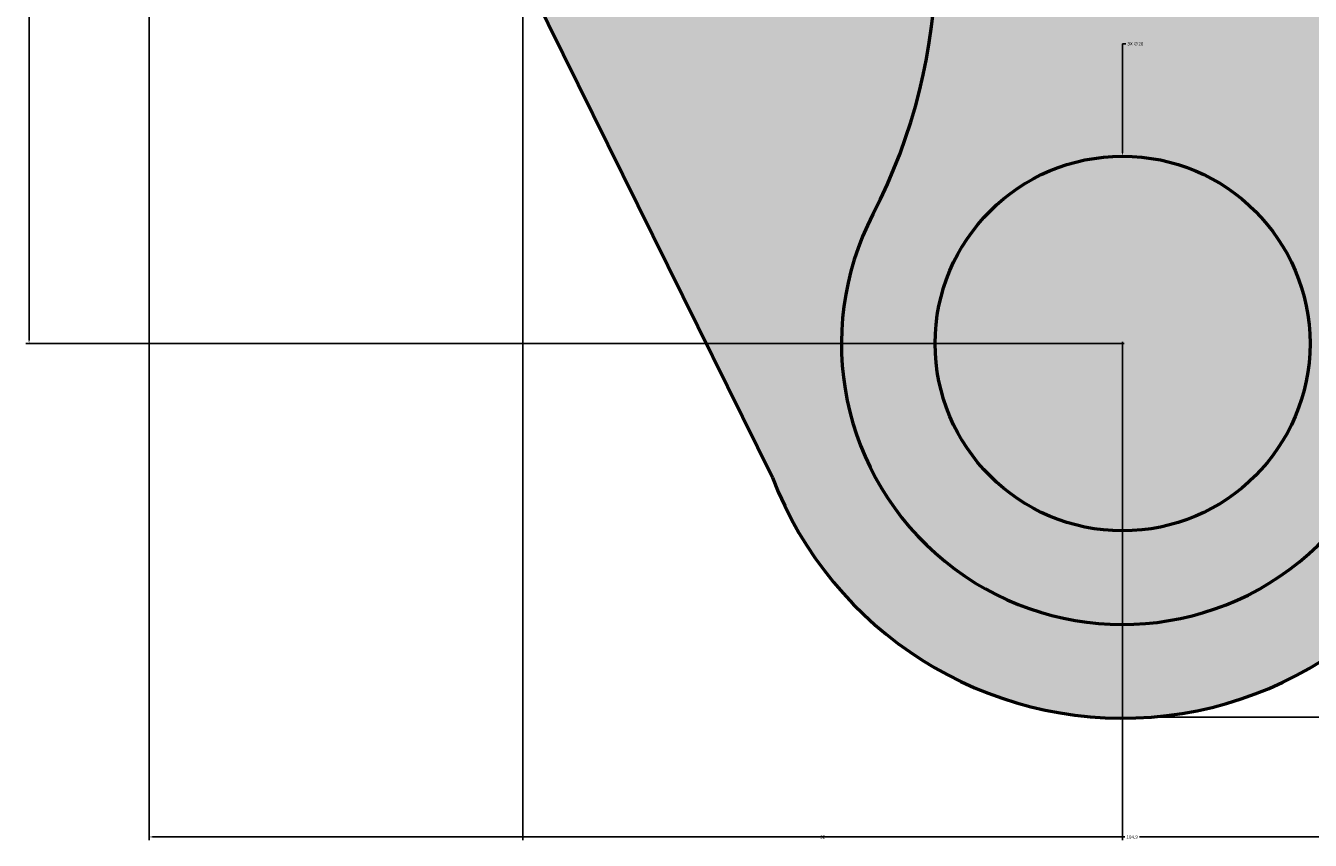
# Model space of a CAD drawing. Units: inches. Extents: x -31 to 87, y -18 to 100.
# Tile 1 of 7: x -31 to 37, y -18 to 25. Entities that reach past the tile are written whole.
import ezdxf

# ---------------------------------------------------------------- set-up
doc = ezdxf.new("R2010")
doc.units = ezdxf.units.IN
doc.header["$MEASUREMENT"] = 0
for name, color, linetype, lineweight in [('M-DIMS', 2, 'Continuous', 18), ('M-HATC', 7, 'Continuous', 18), ('M-OUTL', 4, 'Continuous', 50)]:
    doc.layers.add(name, color=color, linetype=linetype, lineweight=lineweight)
doc.styles.get("Standard").update_dxf_attribs({"font": 'arial.ttf'})
doc.dimstyles.get("Standard").update_dxf_attribs({"dimtxt": 0.18, "dimasz": 0.18, "dimexe": 0.18, "dimexo": 0.0625, "dimgap": 0.09, "dimtad": 0, "dimtih": 1, "dimtoh": 1, "dimdec": 4, "dimzin": 0, "dimdsep": 46, "dimtxsty": 'Standard', "dimcen": 0.09, "dimadec": 0, "dimazin": 0, "dimtfac": 1, "dimtdec": 4, "dimtofl": 0, "dimtmove": 0, "dimatfit": 3, "dimfxl": 1, "dimtolj": 1, "dimtzin": 0, "dimarcsym": 0})

# ---------------------------------------------------------------- blocks, each defined once
blk = doc.blocks.new('*D1')
at = {"layer": 'Defpoints', "color": 0, "transparency": 16777216}
for p in [(-24.622, 75.027), (80.28, 72.235), (80.28, -17.851)]:
    blk.add_point(p, dxfattribs=at)
at = {"layer": 'M-DIMS', "color": 0, "lineweight": -2, "transparency": 16777216}
for p, q in [((-24.622, 74.965), (-24.622, -18.031)), ((80.28, 72.173), (80.28, -18.031)), ((-24.442, -17.851), (27.443, -17.851)), ((80.1, -17.851), (28.214, -17.851))]:
    blk.add_line(p, q, dxfattribs=at)
at = {"layer": 'M-DIMS', "color": 0, "transparency": 16777216}
for points in [[(-24.442, -17.821), (-24.442, -17.881), (-24.622, -17.851)], [(80.1, -17.821), (80.1, -17.881), (80.28, -17.851)]]:
    blk.add_solid(points, dxfattribs=at)
at = {"layer": 'M-DIMS', "color": 0, "transparency": 16777216, "insert": (27.829, -17.851), "char_height": 0.18, "attachment_point": 5}
blk.add_mtext('\\A1;104.9', dxfattribs=at)
blk = doc.blocks.new('*D2')
at = {"layer": 'Defpoints', "color": 0, "transparency": 16777216}
for p in [(60.278, 93.49), (86.68, 93.49), (28.858, -11.451)]:
    blk.add_point(p, dxfattribs=at)
at = {"layer": 'M-DIMS', "color": 0, "lineweight": -2, "transparency": 16777216}
for p, q in [((60.341, 93.49), (86.86, 93.49)), ((86.68, 93.31), (86.68, 41.201)), ((86.68, -11.271), (86.68, 40.838)), ((28.92, -11.451), (86.86, -11.451))]:
    blk.add_line(p, q, dxfattribs=at)
at = {"layer": 'M-DIMS', "color": 0, "transparency": 16777216}
for points in [[(86.65, 93.31), (86.71, 93.31), (86.68, 93.49)], [(86.65, -11.271), (86.71, -11.271), (86.68, -11.451)]]:
    blk.add_solid(points, dxfattribs=at)
at = {"layer": 'M-DIMS', "color": 0, "transparency": 16777216, "insert": (86.68, 41.019), "char_height": 0.18, "attachment_point": 5}
blk.add_mtext('\\A1;104.94', dxfattribs=at)
blk = doc.blocks.new('*D4')
at = {"layer": 'Defpoints', "color": 0, "transparency": 16777216}
for p in [(-4.681, 73.49), (27.319, 8.49), (27.319, -17.851)]:
    blk.add_point(p, dxfattribs=at)
at = {"layer": 'M-DIMS', "color": 0, "lineweight": -2, "transparency": 16777216}
for p, q in [((-4.681, 73.427), (-4.681, -18.031)), ((27.319, 8.427), (27.319, -18.031)), ((-4.501, -17.851), (11.101, -17.851)), ((27.139, -17.851), (11.537, -17.851))]:
    blk.add_line(p, q, dxfattribs=at)
at = {"layer": 'M-DIMS', "color": 0, "transparency": 16777216}
for points in [[(-4.501, -17.821), (-4.501, -17.881), (-4.681, -17.851)], [(27.139, -17.821), (27.139, -17.881), (27.319, -17.851)]]:
    blk.add_solid(points, dxfattribs=at)
at = {"layer": 'M-DIMS', "color": 0, "transparency": 16777216, "insert": (11.319, -17.851), "char_height": 0.18, "attachment_point": 5}
blk.add_mtext('\\A1;32', dxfattribs=at)
blk = doc.blocks.new('*D5')
at = {"layer": 'Defpoints', "color": 0, "transparency": 16777216}
for p in [(-31.022, 73.49), (-4.681, 73.49), (27.319, 8.49)]:
    blk.add_point(p, dxfattribs=at)
at = {"layer": 'M-DIMS', "color": 0, "lineweight": -2, "transparency": 16777216}
for p, q in [((-4.744, 73.49), (-31.202, 73.49)), ((-31.022, 73.31), (-31.022, 41.172)), ((-31.022, 8.67), (-31.022, 40.808)), ((27.256, 8.49), (-31.202, 8.49))]:
    blk.add_line(p, q, dxfattribs=at)
at = {"layer": 'M-DIMS', "color": 0, "transparency": 16777216}
for points in [[(-31.052, 73.31), (-30.992, 73.31), (-31.022, 73.49)], [(-31.052, 8.67), (-30.992, 8.67), (-31.022, 8.49)]]:
    blk.add_solid(points, dxfattribs=at)
at = {"layer": 'M-DIMS', "color": 0, "transparency": 16777216, "insert": (-31.022, 40.99), "char_height": 0.18, "attachment_point": 5}
blk.add_mtext('\\A1;65', dxfattribs=at)
blk = doc.blocks.new('*D6')
at = {"layer": 'Defpoints', "color": 0, "transparency": 16777216}
for p in [(27.319, 18.49), (27.319, -1.51)]:
    blk.add_point(p, dxfattribs=at)
at = {"layer": 'M-DIMS', "color": 0, "lineweight": -2, "transparency": 16777216}
for p, q in [((27.499, 24.49), (27.319, 24.49)), ((27.319, 24.49), (27.319, 18.67)), ((27.229, 8.49), (27.409, 8.49)), ((27.319, 8.4), (27.319, 8.58))]:
    blk.add_line(p, q, dxfattribs=at)
at = {"layer": 'M-DIMS', "color": 0, "transparency": 16777216}
blk.add_solid([(27.289, 18.67), (27.349, 18.67), (27.319, 18.49)], dxfattribs=at)
at = {"layer": 'M-DIMS', "color": 0, "transparency": 16777216, "insert": (28.004, 24.49), "char_height": 0.18, "attachment_point": 5}
blk.add_mtext('\\A1;3X ∅20', dxfattribs=at)

msp = doc.modelspace()

# ---------------------------------------------------------------- hatches: boundary and pattern name
at = {"layer": 'M-HATC'}
h = msp.add_hatch(color=256, dxfattribs=at)
h.set_gradient(color1=(205, 32, 39), color2=(247, 242, 129))
h.paths.add_polyline_path([(-2.425, 93.362, 0.593504), (-22.614, 64.635), (8.64, 1.342, 0.746388), (46.874, 4.293), (79.436, 67.614, 0.505151), (60.278, 93.49)])
h.paths.add_polyline_path([(49.486, 83.865, -1.392259), (62.663, 58.674, 0.510547), (40.663, 15.341, -1.641082), (14.002, 15.393, 0.505248), (-7.332, 58.726, -1.377138), (6.152, 83.865, 0.426931)], flags=16)
h.paths.add_polyline_path([(5.319, 73.49, -1), (-14.681, 73.49, -1)], flags=0)
h.paths.add_polyline_path([(70.319, 73.49, -1), (50.319, 73.49, -1)], flags=0)
h.paths.add_polyline_path([(37.319, 8.49, -1), (17.319, 8.49, -1)], flags=0)
h.paths.add_polyline_path([(6.152, 83.865, 1.377138), (-7.332, 58.726, -0.505248), (14.002, 15.393, 1.641082), (40.663, 15.341, -0.510547), (62.663, 58.674, 1.392259), (49.486, 83.865, -0.426931)], flags=0)
h = msp.add_hatch(color=256, dxfattribs=at)
h.dxf.hatch_style = 1
h.paths.add_polyline_path([(5.319, 73.49, 1), (-14.681, 73.49, 1)])
h.paths.add_polyline_path([(50.319, 73.49, 1), (70.319, 73.49, 1)])
h.paths.add_polyline_path([(37.319, 8.49, 1), (17.319, 8.49, 1)])

# ---------------------------------------------------------------- linework, layer by layer
at = {"layer": 'M-OUTL'}
msp.add_line((8.64, 1.342), (-22.614, 64.635), dxfattribs=at)
msp.add_circle((27.319, 8.49), 10, dxfattribs=at)
for centre, radius, start, end in [((-12.633, 29.198), 30, 332.60114, 79.82161), ((27.319, 8.49), 15, 152.60114, 27.17632), ((27.319, 8.49), 20, 200.93859, 347.88753)]:
    msp.add_arc(centre, radius, start, end, dxfattribs=at)

# ---------------------------------------------------------------- dimensions: what is measured, and where the dimension line sits
at = {"layer": 'M-DIMS'}
for base, p1, p2, override, picture, middle in [((86.68, 93.49), (28.858, -11.451), (60.278, 93.49), {"dimdec": 2, "dimlfac": 1, "dimrnd": 0, "dimzin": 0, "dimdsep": 46, "dimlunit": 2}, '*D2', (86.68, 41.019)), ((-31.022, 73.49), (27.319, 8.49), (-4.681, 73.49), {"dimdec": 0, "dimlfac": 1, "dimrnd": 0, "dimzin": 0, "dimdsep": 46, "dimlunit": 2}, '*D5', (-31.022, 40.99))]:
    dim = msp.add_linear_dim(base=base, p1=p1, p2=p2, angle=90, dimstyle='Standard', override=override, dxfattribs=at)
    dim.commit()
    dim.dimension.update_dxf_attribs({"geometry": picture, "text_midpoint": middle})
for base, p1, p2, override, picture, middle in [((80.28, -17.851), (-24.622, 75.027), (80.28, 72.235), {"dimdec": 1, "dimlfac": 1, "dimrnd": 0, "dimzin": 0, "dimdsep": 46, "dimlunit": 2}, '*D1', (27.829, -17.851)), ((27.319, -17.851), (-4.681, 73.49), (27.319, 8.49), {"dimdec": 0, "dimlfac": 1, "dimrnd": 0, "dimzin": 0, "dimdsep": 46, "dimlunit": 2}, '*D4', (11.319, -17.851))]:
    dim = msp.add_linear_dim(base=base, p1=p1, p2=p2, dimstyle='Standard', override=override, dxfattribs=at)
    dim.commit()
    dim.dimension.update_dxf_attribs({"geometry": picture, "text_midpoint": middle})
dim = msp.add_diameter_dim_2p(p1=(27.319, -1.51), p2=(27.319, 18.49), text='3X <>', dimstyle='Standard', override={"dimdec": 0, "dimlfac": 1, "dimrnd": 0, "dimzin": 0, "dimdsep": 46, "dimlunit": 2}, dxfattribs=at)
dim.commit()
dim.dimension.update_dxf_attribs({"geometry": '*D6', "text_midpoint": (28.004, 24.49), "dimtype": 163})

doc.saveas('drawing.dxf')
